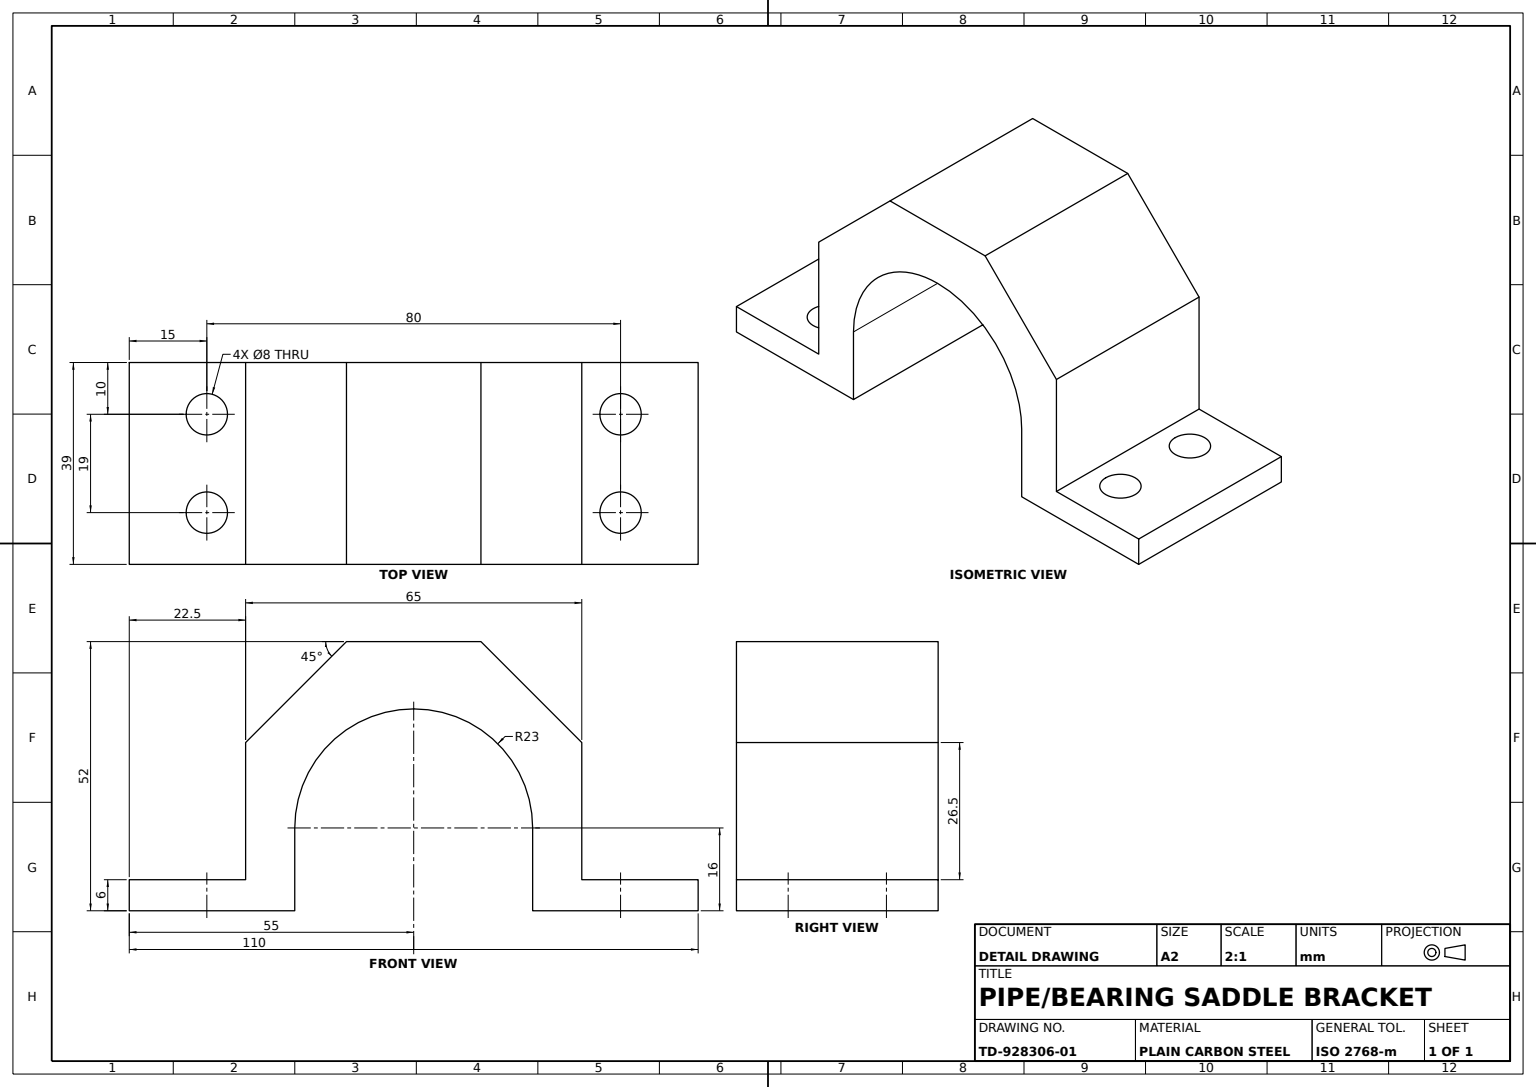
from build123d import *

# Parameters (mm, degrees)
BASE_PLATE_SKETCH_W       = 110
BASE_PLATE_SKETCH_H       = 39
BASE_PLATE_110X39X6_DEPTH = 6
SADDLE_BODY_39_DEPTH      = 39
SADDLE_CUTOUT_SKETCH_W    = 46
SADDLE_CUTOUT_SKETCH_H    = 6
SADDLE_CUTOUT_DEPTH       = 39
FLANGE_HOLES_SKETCH_R     = 4
FLANGE_HOLES_4X_8_DEPTH   = 39


with BuildPart() as part:
    # Base Plate Sketch → Base Plate 110x39x6 (new body)
    with BuildSketch(Plane.XY):
        with Locations((55, 19.5)):
            Rectangle(BASE_PLATE_SKETCH_W, BASE_PLATE_SKETCH_H)
    extrude(amount=BASE_PLATE_110X39X6_DEPTH)

    # Saddle Body Profile → Saddle Body 39 (add)
    with BuildSketch(Plane.XZ):
        with BuildLine():
            Line((32, -10), (32, 0))
            Line((32, 0), (22.5, 0))
            Line((22.5, 0), (22.5, -26.5))
            Line((22.5, -26.5), (42, -46))
            Line((42, -46), (55, -46))
            Line((55, -46), (55, -33))
            ThreePointArc((55, -33), (38.736544033, -26.263455967), (32, -10))
        make_face()
        with BuildLine():
            Line((87.5, 0), (78, 0))
            Line((78, 0), (78, -10))
            ThreePointArc((78, -10), (71.263455967, -26.263455967), (55, -33))
            Line((55, -33), (55, -46))
            Line((55, -46), (68, -46))
            Line((68, -46), (87.5, -26.5))
            Line((87.5, -26.5), (87.5, 0))
        make_face()
    extrude(amount=-SADDLE_BODY_39_DEPTH)

    # Saddle Cutout Sketch → Saddle Cutout (cut)
    with BuildSketch(Plane.XZ):
        with Locations((55, 3)):
            Rectangle(SADDLE_CUTOUT_SKETCH_W, SADDLE_CUTOUT_SKETCH_H)
    extrude(amount=-SADDLE_CUTOUT_DEPTH, mode=Mode.SUBTRACT)

    # Flange Holes Sketch → Flange Holes 4xØ8 (cut)
    with BuildSketch(Plane.XY.offset(6)):
        with Locations((15, 29)):
            Circle(FLANGE_HOLES_SKETCH_R)
        with Locations((15, 10)):
            Circle(FLANGE_HOLES_SKETCH_R)
        with Locations((95, 29)):
            Circle(FLANGE_HOLES_SKETCH_R)
        with Locations((95, 10)):
            Circle(FLANGE_HOLES_SKETCH_R)
    extrude(amount=-FLANGE_HOLES_4X_8_DEPTH, mode=Mode.SUBTRACT)


solid = part.part
